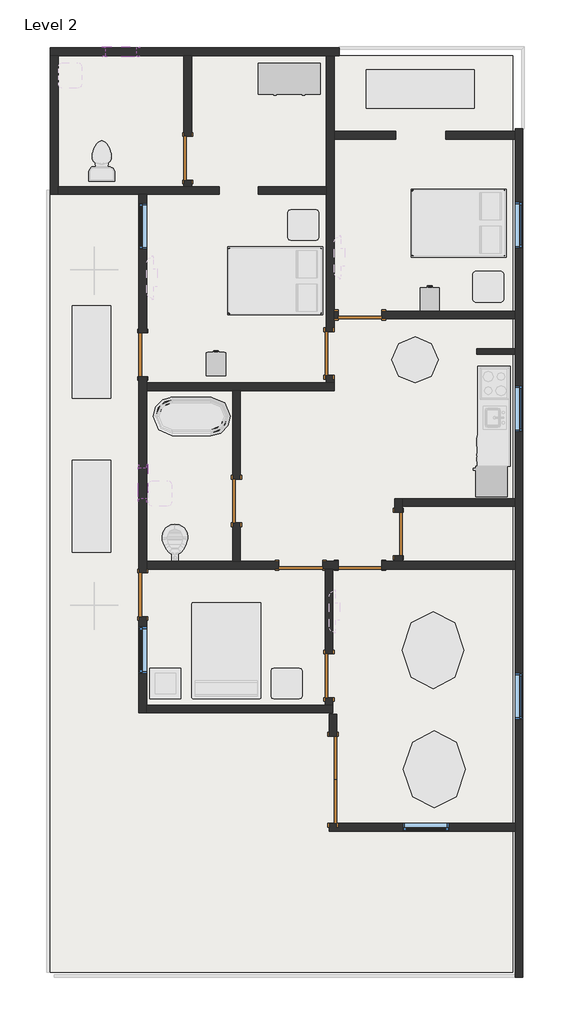
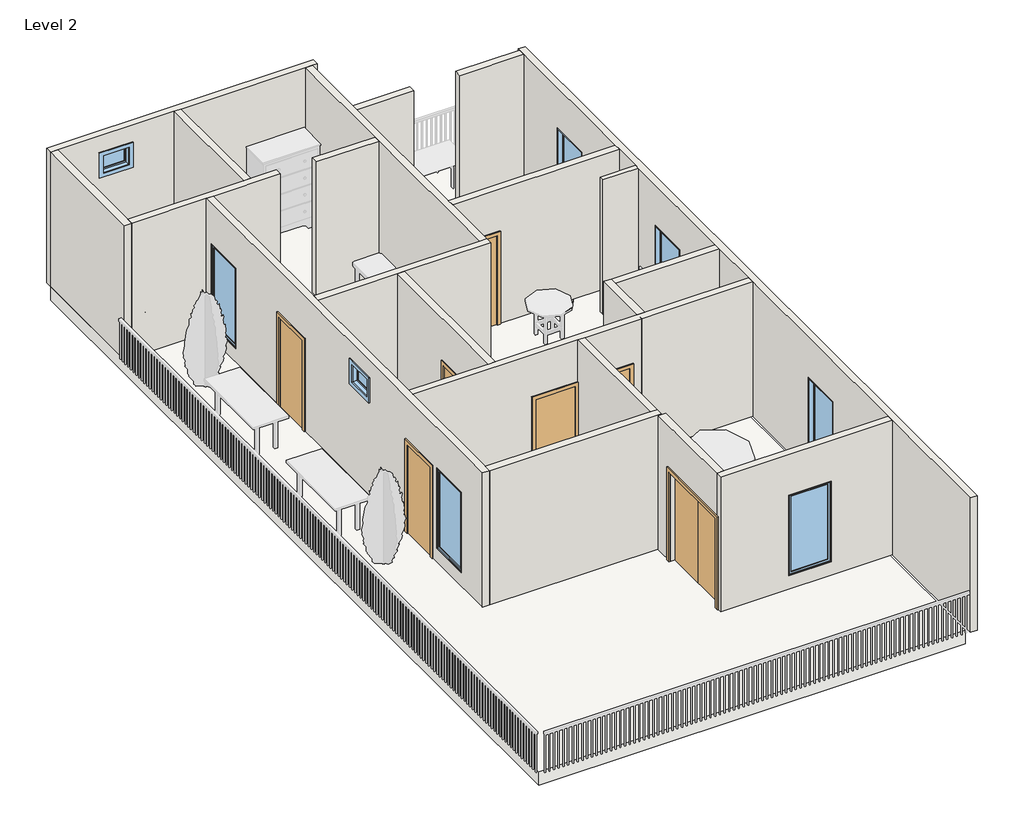
# One storey, part 1 of 4: 22 walls, 11 doors, 8 windows, 1 slab.
"""IFC4 building model written with IfcOpenShell, lengths in millimetres."""

from ifc_helpers import new_model, si_unit, frame, origin, place, context, project, spatial, polyline, outline, extrude, faceted_brep, transform, mapped, element, save
from components import door_74777eb6, door_56e8e0a9, door_706f0888, window_c05a16fb, window_8f6a5eb6

model = new_model("IFC4")

# Units and contexts
model_context = context("Model", 3, world=origin())
ifc_project = project(units=[si_unit("LENGTHUNIT", "METRE", prefix="MILLI")], contexts=[model_context])

# Site, building, storey
site = spatial("IfcSite", under=ifc_project)
building = spatial("IfcBuilding", under=site)
storey = spatial("IfcBuildingStorey", under=building, Name="Level 2", Elevation=3048.0)

# Doors
placement = place(None, origin())
door_shape = door_74777eb6(model_context)
element("IfcDoor", 1, ObjectType="Door-Double-Flush_Panel : 68\" x 80\"", at=placement, inside=storey, context=model_context, shape_type="MappedRepresentation", body=[
    mapped(door_shape, transform((-6447.060887, -797.8089531, 3048.0), x_axis=(0.0, -1.0, 0.0), y_axis=(1.0, 0.0, 0.0), z_axis=(0.0, 0.0, 1.0))),
])
door_2_shape = door_56e8e0a9(model_context)
element("IfcDoor", 2, ObjectType="Single-Flush : 34\" x 80\"", at=placement, inside=storey, context=model_context, shape_type="MappedRepresentation", body=[
    mapped(door_2_shape, transform((-5913.660887, 8396.9910469, 3048.0), x_axis=(-1.0, 0.0, 0.0), y_axis=(0.0, -1.0, 0.0), z_axis=(0.0, 0.0, 1.0))),
])
element("IfcDoor", 3, ObjectType="Single-Flush : 34\" x 80\"", at=placement, inside=storey, context=model_context, shape_type="MappedRepresentation", body=[
    mapped(door_2_shape, transform((-10206.260887, 2859.7910469, 3048.0), x_axis=(0.0, 1.0, 0.0), y_axis=(-1.0, 0.0, 0.0), z_axis=(0.0, 0.0, 1.0))),
])
element("IfcDoor", 4, ObjectType="Single-Flush : 34\" x 80\"", at=placement, inside=storey, context=model_context, shape_type="MappedRepresentation", body=[
    mapped(door_2_shape, transform((-5151.660887, 4066.2910469, 3048.0), x_axis=(0.0, -1.0, 0.0), y_axis=(1.0, 0.0, 0.0), z_axis=(0.0, 0.0, 1.0))),
])
element("IfcDoor", 5, ObjectType="Single-Flush : 34\" x 80\"", at=placement, inside=storey, context=model_context, shape_type="MappedRepresentation", body=[
    mapped(door_2_shape, transform((-5913.660887, 3443.9910469, 3048.0), x_axis=(-1.0, 0.0, 0.0), y_axis=(0.0, -1.0, 0.0), z_axis=(0.0, 0.0, 1.0))),
])
door_3_shape = door_706f0888(model_context)
element("IfcDoor", 6, ObjectType="Single-Flush : 34\" x 80\"", at=placement, inside=storey, context=model_context, shape_type="MappedRepresentation", body=[
    mapped(door_3_shape, transform((-9317.260887, 11495.7910469, 3048.0), x_axis=(0.0, -1.0, 0.0), y_axis=(1.0, 0.0, 0.0), z_axis=(0.0, 0.0, 1.0))),
])
element("IfcDoor", 7, ObjectType="Single-Flush : 34\" x 80\"", at=placement, inside=storey, context=model_context, shape_type="MappedRepresentation", body=[
    mapped(door_3_shape, transform((-6523.260887, 7634.9910469, 3048.0), x_axis=(0.0, -1.0, 0.0), y_axis=(1.0, 0.0, 0.0), z_axis=(0.0, 0.0, 1.0))),
])
element("IfcDoor", 8, ObjectType="Single-Flush : 34\" x 80\"", at=placement, inside=storey, context=model_context, shape_type="MappedRepresentation", body=[
    mapped(door_3_shape, transform((-8352.060887, 4713.9910469, 3048.0), x_axis=(0.0, -1.0, 0.0), y_axis=(1.0, 0.0, 0.0), z_axis=(0.0, 0.0, 1.0))),
])
element("IfcDoor", 9, ObjectType="Single-Flush : 34\" x 80\"", at=placement, inside=storey, context=model_context, shape_type="MappedRepresentation", body=[
    mapped(door_3_shape, transform((-7082.060887, 3443.9910469, 3048.0), x_axis=(1.0, 0.0, 0.0), y_axis=(0.0, 1.0, 0.0), z_axis=(0.0, 0.0, 1.0))),
])
element("IfcDoor", 10, ObjectType="Single-Flush : 34\" x 80\"", at=placement, inside=storey, context=model_context, shape_type="MappedRepresentation", body=[
    mapped(door_3_shape, transform((-10206.260887, 7609.5910469, 3048.0), x_axis=(0.0, -1.0, 0.0), y_axis=(1.0, 0.0, 0.0), z_axis=(0.0, 0.0, 1.0))),
])
element("IfcDoor", 11, ObjectType="Single-Flush : 34\" x 80\"", at=placement, inside=storey, context=model_context, shape_type="MappedRepresentation", body=[
    mapped(door_3_shape, transform((-6523.260887, 1259.5910469, 3048.0), x_axis=(0.0, -1.0, 0.0), y_axis=(1.0, 0.0, 0.0), z_axis=(0.0, 0.0, 1.0))),
])

# Slab
element("IfcSlab", 12, ObjectType="Generic - 12\"", at=placement, inside=storey, context=model_context, shape_type="SweptSolid", body=[
    extrude(outline(polyline([(-2891.060887, 13527.7910469), (-2891.060887, -4607.8089531), (-12035.060887, -4607.8089531), (-12035.060887, 13527.7910469), (-2891.060887, 13527.7910469)])), frame((0.0, 0.0, 2743.2), z_axis=(0.0, 0.0, 1.0), x_axis=(1.0, 0.0, 0.0)), (0.0, 0.0, 1.0), 304.8),
])

# Walls
element("IfcWall", 13, ObjectType="Generic - 8\"", at=placement, inside=storey, context=model_context, shape_type="Brep", body=[
    faceted_brep([(-12035.060887, 13527.7910469, 3048.0), (-11882.660887, 13527.7910469, 3048.0), (-9393.460887, 13527.7910469, 3048.0), (-9241.060887, 13527.7910469, 3048.0), (-6574.060887, 13527.7910469, 3048.0), (-6421.660887, 13527.7910469, 3048.0), (-6320.060887, 13527.7910469, 3048.0), (-6320.060887, 13527.7910469, 6096.0), (-6421.660887, 13527.7910469, 6096.0), (-6574.060887, 13527.7910469, 6096.0), (-9241.060887, 13527.7910469, 6096.0), (-9393.460887, 13527.7910469, 6096.0), (-11882.660887, 13527.7910469, 6096.0), (-12035.060887, 13527.7910469, 6096.0), (-10333.260887, 13527.7910469, 5664.2), (-10333.260887, 13527.7910469, 5207.0), (-10942.860887, 13527.7910469, 5207.0), (-10942.860887, 13527.7910469, 5664.2), (-12035.060887, 13680.1910469, 3048.0), (-12035.060887, 13680.1910469, 6096.0), (-6320.060887, 13680.1910469, 6096.0), (-6320.060887, 13680.1910469, 3048.0), (-10333.260887, 13680.1910469, 5664.2), (-10942.860887, 13680.1910469, 5664.2), (-10942.860887, 13680.1910469, 5207.0), (-10333.260887, 13680.1910469, 5207.0)], [[[0, 1, 2, 3, 4, 5, 6, 7, 8, 9, 10, 11, 12, 13], [14, 15, 16, 17]], [[18, 19, 20, 21], [22, 23, 24, 25]], [[6, 5, 4, 3, 2, 1, 0, 18, 21]], [[7, 6, 21, 20]], [[13, 12, 11, 10, 9, 8, 7, 20, 19]], [[0, 13, 19, 18]], [[15, 14, 22, 25]], [[16, 15, 25, 24]], [[17, 16, 24, 23]], [[14, 17, 23, 22]]]),
])
element("IfcWall", 14, ObjectType="Generic - 8\"", at=placement, inside=storey, context=model_context, shape_type="Brep", body=[
    faceted_brep([(-12035.060887, 13527.7910469, 3048.0), (-12035.060887, 10784.5910469, 3048.0), (-12035.060887, 10784.5910469, 6096.0), (-12035.060887, 13527.7910469, 6096.0), (-11882.660887, 13527.7910469, 3048.0), (-11882.660887, 13527.7910469, 6096.0), (-11882.660887, 10936.9910469, 6096.0), (-11882.660887, 10784.5910469, 6096.0), (-11882.660887, 10784.5910469, 3048.0), (-11882.660887, 10936.9910469, 3048.0)], [[[0, 1, 2, 3]], [[4, 5, 6, 7, 8, 9]], [[1, 0, 4, 9, 8]], [[3, 2, 7, 6, 5]], [[0, 3, 5, 4]], [[2, 1, 8, 7]]]),
])
element("IfcWall", 15, ObjectType="Generic - 8\"", at=placement, inside=storey, context=model_context, shape_type="Brep", body=[
    faceted_brep([(-11882.660887, 10784.5910469, 3048.0), (-10282.460887, 10784.5910469, 3048.0), (-10130.060887, 10784.5910469, 3048.0), (-8694.960887, 10784.5910469, 3048.0), (-8694.960887, 10784.5910469, 6096.0), (-10130.060887, 10784.5910469, 6096.0), (-10282.460887, 10784.5910469, 6096.0), (-11882.660887, 10784.5910469, 6096.0), (-11882.660887, 10936.9910469, 3048.0), (-11882.660887, 10936.9910469, 6096.0), (-9393.460887, 10936.9910469, 6096.0), (-9241.060887, 10936.9910469, 6096.0), (-8694.960887, 10936.9910469, 6096.0), (-8694.960887, 10936.9910469, 3048.0), (-9241.060887, 10936.9910469, 3048.0), (-9393.460887, 10936.9910469, 3048.0)], [[[0, 1, 2, 3, 4, 5, 6, 7]], [[8, 9, 10, 11, 12, 13, 14, 15]], [[3, 2, 1, 0, 8, 15, 14, 13]], [[4, 3, 13, 12]], [[7, 6, 5, 4, 12, 11, 10, 9]], [[0, 7, 9, 8]]]),
])
element("IfcWall", 16, ObjectType="Generic - 8\"", at=placement, inside=storey, context=model_context, shape_type="Brep", body=[
    faceted_brep([(-10282.460887, 522.9910469, 6096.0), (-10282.460887, 10784.5910469, 6096.0), (-10282.460887, 10784.5910469, 3048.0), (-10282.460887, 8041.3910469, 3048.0), (-10282.460887, 8041.3910469, 5080.0), (-10282.460887, 7177.7910469, 5080.0), (-10282.460887, 7177.7910469, 3048.0), (-10282.460887, 3291.5910469, 3048.0), (-10282.460887, 3291.5910469, 5080.0), (-10282.460887, 2427.9910469, 5080.0), (-10282.460887, 2427.9910469, 3048.0), (-10282.460887, 522.9910469, 3048.0), (-10282.460887, 10606.7910469, 3352.8), (-10282.460887, 10606.7910469, 5181.6), (-10282.460887, 9692.3910469, 5181.6), (-10282.460887, 9692.3910469, 3352.8), (-10282.460887, 2224.7910469, 3352.8), (-10282.460887, 2224.7910469, 5181.6), (-10282.460887, 1310.3910469, 5181.6), (-10282.460887, 1310.3910469, 3352.8), (-10282.460887, 4764.7910469, 5664.2), (-10282.460887, 4764.7910469, 5207.0), (-10282.460887, 5374.3910469, 5207.0), (-10282.460887, 5374.3910469, 5664.2), (-10130.060887, 10784.5910469, 6096.0), (-10130.060887, 7050.7910469, 6096.0), (-10130.060887, 6898.3910469, 6096.0), (-10130.060887, 3520.1910469, 6096.0), (-10130.060887, 3367.7910469, 6096.0), (-10130.060887, 675.3910469, 6096.0), (-10130.060887, 522.9910469, 6096.0), (-10130.060887, 522.9910469, 3048.0), (-10130.060887, 675.3910469, 3048.0), (-10130.060887, 2427.9910469, 3048.0), (-10130.060887, 2427.9910469, 5080.0), (-10130.060887, 3291.5910469, 5080.0), (-10130.060887, 3291.5910469, 3048.0), (-10130.060887, 3367.7910469, 3048.0), (-10130.060887, 3520.1910469, 3048.0), (-10130.060887, 6898.3910469, 3048.0), (-10130.060887, 7050.7910469, 3048.0), (-10130.060887, 7177.7910469, 3048.0), (-10130.060887, 7177.7910469, 5080.0), (-10130.060887, 8041.3910469, 5080.0), (-10130.060887, 8041.3910469, 3048.0), (-10130.060887, 10784.5910469, 3048.0), (-10130.060887, 10606.7910469, 5181.6), (-10130.060887, 10606.7910469, 3352.8), (-10130.060887, 9692.3910469, 3352.8), (-10130.060887, 9692.3910469, 5181.6), (-10130.060887, 2224.7910469, 5181.6), (-10130.060887, 2224.7910469, 3352.8), (-10130.060887, 1310.3910469, 3352.8), (-10130.060887, 1310.3910469, 5181.6), (-10130.060887, 4764.7910469, 5207.0), (-10130.060887, 4764.7910469, 5664.2), (-10130.060887, 5374.3910469, 5664.2), (-10130.060887, 5374.3910469, 5207.0)], [[[0, 1, 2, 3, 4, 5, 6, 7, 8, 9, 10, 11], [12, 13, 14, 15], [16, 17, 18, 19], [20, 21, 22, 23]], [[24, 25, 26, 27, 28, 29, 30, 31, 32, 33, 34, 35, 36, 37, 38, 39, 40, 41, 42, 43, 44, 45], [46, 47, 48, 49], [50, 51, 52, 53], [54, 55, 56, 57]], [[2, 45, 44, 3]], [[31, 11, 10, 33, 32]], [[6, 41, 40, 39, 38, 37, 36, 7]], [[1, 0, 30, 29, 28, 27, 26, 25, 24]], [[2, 1, 24, 45]], [[0, 11, 31, 30]], [[12, 47, 46, 13]], [[47, 12, 15, 48]], [[48, 15, 14, 49]], [[50, 17, 16, 51]], [[51, 16, 19, 52]], [[52, 19, 18, 53]], [[13, 46, 49, 14]], [[17, 50, 53, 18]], [[21, 20, 55, 54]], [[22, 21, 54, 57]], [[23, 22, 57, 56]], [[20, 23, 56, 55]], [[42, 41, 6, 5]], [[43, 42, 5, 4]], [[44, 43, 4, 3]], [[35, 8, 7, 36]], [[8, 35, 34, 9]], [[10, 9, 34, 33]]]),
])
element("IfcWall", 17, ObjectType="Generic - 8\"", at=placement, inside=storey, context=model_context, shape_type="Brep", body=[
    faceted_brep([(-10130.060887, 6898.3910469, 3048.0), (-8428.260887, 6898.3910469, 3048.0), (-8275.860887, 6898.3910469, 3048.0), (-6421.660887, 6898.3910469, 3048.0), (-6421.660887, 6898.3910469, 6096.0), (-8275.860887, 6898.3910469, 6096.0), (-8428.260887, 6898.3910469, 6096.0), (-10130.060887, 6898.3910469, 6096.0), (-10130.060887, 7050.7910469, 3048.0), (-10130.060887, 7050.7910469, 6096.0), (-6574.060887, 7050.7910469, 6096.0), (-6421.660887, 7050.7910469, 6096.0), (-6421.660887, 7050.7910469, 3048.0), (-6574.060887, 7050.7910469, 3048.0)], [[[0, 1, 2, 3, 4, 5, 6, 7]], [[8, 9, 10, 11, 12, 13]], [[3, 2, 1, 0, 8, 13, 12]], [[7, 6, 5, 4, 11, 10, 9]], [[0, 7, 9, 8]], [[4, 3, 12, 11]]]),
])
element("IfcWall", 18, ObjectType="Generic - 8\"", at=placement, inside=storey, context=model_context, shape_type="Brep", body=[
    faceted_brep([(-6421.660887, 13527.7910469, 6096.0), (-6421.660887, 12029.1910469, 6096.0), (-6421.660887, 11876.7910469, 6096.0), (-6421.660887, 8473.1910469, 6096.0), (-6421.660887, 8320.7910469, 6096.0), (-6421.660887, 7050.7910469, 6096.0), (-6421.660887, 7050.7910469, 3048.0), (-6421.660887, 7203.1910469, 3048.0), (-6421.660887, 7203.1910469, 5080.0), (-6421.660887, 8066.7910469, 5080.0), (-6421.660887, 8066.7910469, 3048.0), (-6421.660887, 8320.7910469, 3048.0), (-6421.660887, 8473.1910469, 3048.0), (-6421.660887, 11876.7910469, 3048.0), (-6421.660887, 12029.1910469, 3048.0), (-6421.660887, 13527.7910469, 3048.0), (-6574.060887, 7050.7910469, 6096.0), (-6574.060887, 10784.5910469, 6096.0), (-6574.060887, 10936.9910469, 6096.0), (-6574.060887, 13527.7910469, 6096.0), (-6574.060887, 13527.7910469, 3048.0), (-6574.060887, 10936.9910469, 3048.0), (-6574.060887, 10784.5910469, 3048.0), (-6574.060887, 8066.7910469, 3048.0), (-6574.060887, 8066.7910469, 5080.0), (-6574.060887, 7203.1910469, 5080.0), (-6574.060887, 7203.1910469, 3048.0), (-6574.060887, 7050.7910469, 3048.0)], [[[0, 1, 2, 3, 4, 5, 6, 7, 8, 9, 10, 11, 12, 13, 14, 15]], [[16, 17, 18, 19, 20, 21, 22, 23, 24, 25, 26, 27]], [[6, 27, 26, 7]], [[20, 15, 14, 13, 12, 11, 10, 23, 22, 21]], [[5, 4, 3, 2, 1, 0, 19, 18, 17, 16]], [[6, 5, 16, 27]], [[0, 15, 20, 19]], [[25, 8, 7, 26]], [[8, 25, 24, 9]], [[9, 24, 23, 10]]]),
])
element("IfcWall", 19, ObjectType="Generic - 8\"", at=placement, inside=storey, context=model_context, shape_type="SweptSolid", body=[
    extrude(outline(polyline([(-5202.460887, 11876.7910469), (-6421.660887, 11876.7910469), (-6421.660887, 12029.1910469), (-5202.460887, 12029.1910469), (-5202.460887, 11876.7910469)])), frame((0.0, 0.0, 3048.0), z_axis=(0.0, 0.0, 1.0), x_axis=(1.0, 0.0, 0.0)), (0.0, 0.0, 1.0), 3048.0),
])
element("IfcWall", 20, ObjectType="Generic - 8\"", at=placement, inside=storey, context=model_context, shape_type="SweptSolid", body=[
    extrude(outline(polyline([(3048.0, -6421.660887), (3048.0, -6345.460887), (5080.0, -6345.460887), (5080.0, -5481.860887), (3048.0, -5481.860887), (3048.0, -2840.260887), (6096.0, -2840.260887), (6096.0, -6421.660887), (3048.0, -6421.660887)])), frame((0.0, 8320.7910469, 0.0), z_axis=(0.0, 1.0, 0.0), x_axis=(0.0, 0.0, 1.0)), (0.0, 0.0, 1.0), 152.4),
])
element("IfcWall", 21, ObjectType="Generic - 8\"", at=placement, inside=storey, context=model_context, shape_type="Brep", body=[
    faceted_brep([(-10130.060887, 522.9910469, 3048.0), (-6447.060887, 522.9910469, 3048.0), (-6447.060887, 522.9910469, 6096.0), (-10130.060887, 522.9910469, 6096.0), (-10130.060887, 675.3910469, 3048.0), (-10130.060887, 675.3910469, 6096.0), (-6599.460887, 675.3910469, 6096.0), (-6447.060887, 675.3910469, 6096.0), (-6447.060887, 675.3910469, 3048.0), (-6599.460887, 675.3910469, 3048.0)], [[[0, 1, 2, 3]], [[4, 5, 6, 7, 8, 9]], [[1, 0, 4, 9, 8]], [[3, 2, 7, 6, 5]], [[0, 3, 5, 4]], [[2, 1, 8, 7]]]),
])
element("IfcWall", 22, ObjectType="Generic - 8\"", at=placement, inside=storey, context=model_context, shape_type="SweptSolid", body=[
    extrude(outline(polyline([(827.7910469, 5080.0), (827.7910469, 3048.0), (675.3910469, 3048.0), (675.3910469, 6096.0), (3367.7910469, 6096.0), (3367.7910469, 3048.0), (1691.3910469, 3048.0), (1691.3910469, 5080.0), (827.7910469, 5080.0)])), frame((-6599.460887, 0.0, 0.0), z_axis=(1.0, 0.0, 0.0), x_axis=(0.0, 1.0, 0.0)), (0.0, 0.0, 1.0), 152.4),
])
element("IfcWall", 23, ObjectType="Generic - 8\"", at=placement, inside=storey, context=model_context, shape_type="Brep", body=[
    faceted_brep([(-6345.460887, 3520.1910469, 5080.0), (-6345.460887, 3520.1910469, 3048.0), (-6650.260887, 3520.1910469, 3048.0), (-6650.260887, 3520.1910469, 5080.0), (-7513.860887, 3520.1910469, 5080.0), (-7513.860887, 3520.1910469, 3048.0), (-8275.860887, 3520.1910469, 3048.0), (-8428.260887, 3520.1910469, 3048.0), (-10130.060887, 3520.1910469, 3048.0), (-10130.060887, 3520.1910469, 6096.0), (-8428.260887, 3520.1910469, 6096.0), (-8275.860887, 3520.1910469, 6096.0), (-2840.260887, 3520.1910469, 6096.0), (-2840.260887, 3520.1910469, 3048.0), (-5481.860887, 3520.1910469, 3048.0), (-5481.860887, 3520.1910469, 5080.0), (-6650.260887, 3367.7910469, 3048.0), (-6599.460887, 3367.7910469, 3048.0), (-6447.060887, 3367.7910469, 3048.0), (-6345.460887, 3367.7910469, 3048.0), (-6345.460887, 3367.7910469, 5080.0), (-5481.860887, 3367.7910469, 5080.0), (-5481.860887, 3367.7910469, 3048.0), (-2840.260887, 3367.7910469, 3048.0), (-2840.260887, 3367.7910469, 6096.0), (-6447.060887, 3367.7910469, 6096.0), (-6599.460887, 3367.7910469, 6096.0), (-10130.060887, 3367.7910469, 6096.0), (-10130.060887, 3367.7910469, 3048.0), (-7513.860887, 3367.7910469, 3048.0), (-7513.860887, 3367.7910469, 5080.0), (-6650.260887, 3367.7910469, 5080.0)], [[[0, 1, 2, 3, 4, 5, 6, 7, 8, 9, 10, 11, 12, 13, 14, 15]], [[16, 17, 18, 19, 20, 21, 22, 23, 24, 25, 26, 27, 28, 29, 30, 31]], [[29, 28, 8, 7, 6, 5]], [[14, 13, 23, 22]], [[2, 1, 19, 18, 17, 16]], [[12, 11, 10, 9, 27, 26, 25, 24]], [[9, 8, 28, 27]], [[13, 12, 24, 23]], [[3, 2, 16, 31]], [[4, 3, 31, 30]], [[5, 4, 30, 29]], [[20, 19, 1, 0]], [[21, 20, 0, 15]], [[22, 21, 15, 14]]]),
])
element("IfcWall", 24, ObjectType="Generic - 8\"", at=placement, inside=storey, context=model_context, shape_type="SweptSolid", body=[
    extrude(outline(polyline([(4282.1910469, 5080.0), (4282.1910469, 3048.0), (3520.1910469, 3048.0), (3520.1910469, 6096.0), (6898.3910469, 6096.0), (6898.3910469, 3048.0), (5145.7910469, 3048.0), (5145.7910469, 5080.0), (4282.1910469, 5080.0)])), frame((-8428.260887, 0.0, 0.0), z_axis=(1.0, 0.0, 0.0), x_axis=(0.0, 1.0, 0.0)), (0.0, 0.0, 1.0), 152.4),
])
element("IfcWall", 25, ObjectType="Generic - 8\"", at=placement, inside=storey, context=model_context, shape_type="Brep", body=[
    faceted_brep([(-6523.260887, -1813.8089531, 3048.0), (-2840.260887, -1813.8089531, 3048.0), (-2840.260887, -1813.8089531, 6096.0), (-6523.260887, -1813.8089531, 6096.0), (-5062.760887, -1813.8089531, 3352.8), (-5062.760887, -1813.8089531, 5181.6), (-4148.360887, -1813.8089531, 5181.6), (-4148.360887, -1813.8089531, 3352.8), (-2840.260887, -1661.4089531, 3048.0), (-6523.260887, -1661.4089531, 3048.0), (-6523.260887, -1661.4089531, 5080.0), (-6523.260887, -1661.4089531, 6096.0), (-6370.860887, -1661.4089531, 6096.0), (-2840.260887, -1661.4089531, 6096.0), (-5062.760887, -1661.4089531, 5181.6), (-5062.760887, -1661.4089531, 3352.8), (-4148.360887, -1661.4089531, 3352.8), (-4148.360887, -1661.4089531, 5181.6)], [[[0, 1, 2, 3], [4, 5, 6, 7]], [[8, 9, 10, 11, 12, 13], [14, 15, 16, 17]], [[1, 0, 9, 8]], [[3, 2, 13, 12, 11]], [[2, 1, 8, 13]], [[0, 3, 11, 10, 9]], [[14, 5, 4, 15]], [[15, 4, 7, 16]], [[16, 7, 6, 17]], [[5, 14, 17, 6]]]),
])
element("IfcWall", 26, ObjectType="Generic - 8\"", at=placement, inside=storey, context=model_context, shape_type="SweptSolid", body=[
    extrude(outline(polyline([(497.5910469, 6096.0), (497.5910469, 3048.0), (65.7910469, 3048.0), (65.7910469, 5080.0), (-1661.4089531, 5080.0), (-1661.4089531, 6096.0), (497.5910469, 6096.0)])), frame((-6523.260887, 0.0, 0.0), z_axis=(1.0, 0.0, 0.0), x_axis=(0.0, 1.0, 0.0)), (0.0, 0.0, 1.0), 152.4),
])
element("IfcWall", 27, ObjectType="Generic - 8\"", at=placement, inside=storey, context=model_context, shape_type="Brep", body=[
    faceted_brep([(-2840.260887, 3520.1910469, 3048.0), (-5075.460887, 3520.1910469, 3048.0), (-5227.860887, 3520.1910469, 3048.0), (-5227.860887, 3520.1910469, 6096.0), (-5075.460887, 3520.1910469, 6096.0), (-2840.260887, 3520.1910469, 6096.0), (-2840.260887, 3367.7910469, 3048.0), (-2840.260887, 3367.7910469, 6096.0), (-5227.860887, 3367.7910469, 6096.0), (-5227.860887, 3367.7910469, 3048.0)], [[[0, 1, 2, 3, 4, 5]], [[6, 7, 8, 9]], [[2, 1, 0, 6, 9]], [[5, 4, 3, 8, 7]], [[0, 5, 7, 6]], [[3, 2, 9, 8]]]),
])
element("IfcWall", 28, ObjectType="Generic - 8\"", at=placement, inside=storey, context=model_context, shape_type="Brep", body=[
    faceted_brep([(-5075.460887, 3520.1910469, 3048.0), (-5075.460887, 3634.4910469, 3048.0), (-5075.460887, 3634.4910469, 5080.0), (-5075.460887, 4498.0910469, 5080.0), (-5075.460887, 4498.0910469, 3048.0), (-5075.460887, 4612.3910469, 3048.0), (-5075.460887, 4764.7910469, 3048.0), (-5075.460887, 4764.7910469, 6096.0), (-5075.460887, 4612.3910469, 6096.0), (-5075.460887, 3520.1910469, 6096.0), (-5227.860887, 3634.4910469, 5080.0), (-5227.860887, 3634.4910469, 3048.0), (-5227.860887, 3520.1910469, 3048.0), (-5227.860887, 3520.1910469, 6096.0), (-5227.860887, 4764.7910469, 6096.0), (-5227.860887, 4764.7910469, 3048.0), (-5227.860887, 4498.0910469, 3048.0), (-5227.860887, 4498.0910469, 5080.0)], [[[0, 1, 2, 3, 4, 5, 6, 7, 8, 9]], [[10, 11, 12, 13, 14, 15, 16, 17]], [[16, 15, 6, 5, 4]], [[12, 11, 1, 0]], [[9, 8, 7, 14, 13]], [[0, 9, 13, 12]], [[7, 6, 15, 14]], [[2, 1, 11, 10]], [[3, 2, 10, 17]], [[4, 3, 17, 16]]]),
])
element("IfcWall", 29, ObjectType="Generic - 8\"", at=placement, inside=storey, context=model_context, shape_type="SweptSolid", body=[
    extrude(outline(polyline([(-2840.260887, 4612.3910469), (-5075.460887, 4612.3910469), (-5075.460887, 4764.7910469), (-2840.260887, 4764.7910469), (-2840.260887, 4612.3910469)])), frame((0.0, 0.0, 3048.0), z_axis=(0.0, 0.0, 1.0), x_axis=(1.0, 0.0, 0.0)), (0.0, 0.0, 1.0), 3048.0),
])
element("IfcWall", 30, ObjectType="Generic - 8\"", at=placement, inside=storey, context=model_context, shape_type="SweptSolid", body=[
    extrude(outline(polyline([(10936.9910469, 6096.0), (13527.7910469, 6096.0), (13527.7910469, 3048.0), (11927.5910469, 3048.0), (11927.5910469, 5080.0), (11063.9910469, 5080.0), (11063.9910469, 3048.0), (10936.9910469, 3048.0), (10936.9910469, 6096.0)])), frame((-9393.460887, 0.0, 0.0), z_axis=(1.0, 0.0, 0.0), x_axis=(0.0, 1.0, 0.0)), (0.0, 0.0, 1.0), 152.4),
])
element("IfcWall", 31, ObjectType="Generic - 8\"", at=placement, inside=storey, context=model_context, shape_type="SweptSolid", body=[
    extrude(outline(polyline([(-6574.060887, 10784.5910469), (-7920.260887, 10784.5910469), (-7920.260887, 10936.9910469), (-6574.060887, 10936.9910469), (-6574.060887, 10784.5910469)])), frame((0.0, 0.0, 3048.0), z_axis=(0.0, 0.0, 1.0), x_axis=(1.0, 0.0, 0.0)), (0.0, 0.0, 1.0), 3048.0),
])
element("IfcWall", 32, ObjectType="Generic - 8\"", at=placement, inside=storey, context=model_context, shape_type="SweptSolid", body=[
    extrude(outline(polyline([(-2840.260887, 11876.7910469), (-4211.860887, 11876.7910469), (-4211.860887, 12029.1910469), (-2840.260887, 12029.1910469), (-2840.260887, 11876.7910469)])), frame((0.0, 0.0, 3048.0), z_axis=(0.0, 0.0, 1.0), x_axis=(1.0, 0.0, 0.0)), (0.0, 0.0, 1.0), 3048.0),
])
element("IfcWall", 33, ObjectType="Generic - 8\"", at=placement, inside=storey, context=model_context, shape_type="Brep", body=[
    faceted_brep([(-2840.260887, 12079.9910469, 3048.0), (-2840.260887, 12029.1910469, 3048.0), (-2840.260887, 11876.7910469, 3048.0), (-2840.260887, 8473.1910469, 3048.0), (-2840.260887, 8320.7910469, 3048.0), (-2840.260887, 7723.8910469, 3048.0), (-2840.260887, 7622.2910469, 3048.0), (-2840.260887, 4764.7910469, 3048.0), (-2840.260887, 4612.3910469, 3048.0), (-2840.260887, 3520.1910469, 3048.0), (-2840.260887, 3367.7910469, 3048.0), (-2840.260887, -1661.4089531, 3048.0), (-2840.260887, -1813.8089531, 3048.0), (-2840.260887, -4709.4089531, 3048.0), (-2840.260887, -4709.4089531, 6096.0), (-2840.260887, -1813.8089531, 6096.0), (-2840.260887, -1661.4089531, 6096.0), (-2840.260887, 3367.7910469, 6096.0), (-2840.260887, 3520.1910469, 6096.0), (-2840.260887, 4612.3910469, 6096.0), (-2840.260887, 4764.7910469, 6096.0), (-2840.260887, 7622.2910469, 6096.0), (-2840.260887, 7723.8910469, 6096.0), (-2840.260887, 8320.7910469, 6096.0), (-2840.260887, 8473.1910469, 6096.0), (-2840.260887, 11876.7910469, 6096.0), (-2840.260887, 12029.1910469, 6096.0), (-2840.260887, 12079.9910469, 6096.0), (-2840.260887, 9717.7910469, 5181.6), (-2840.260887, 9717.7910469, 3352.8), (-2840.260887, 10632.1910469, 3352.8), (-2840.260887, 10632.1910469, 5181.6), (-2840.260887, 6085.5910469, 5181.6), (-2840.260887, 6085.5910469, 3352.8), (-2840.260887, 6999.9910469, 3352.8), (-2840.260887, 6999.9910469, 5181.6), (-2840.260887, 395.9910469, 5181.6), (-2840.260887, 395.9910469, 3352.8), (-2840.260887, 1310.3910469, 3352.8), (-2840.260887, 1310.3910469, 5181.6), (-2687.860887, -4709.4089531, 3048.0), (-2687.860887, 12079.9910469, 3048.0), (-2687.860887, 12079.9910469, 6096.0), (-2687.860887, -4709.4089531, 6096.0), (-2687.860887, 9717.7910469, 3352.8), (-2687.860887, 9717.7910469, 5181.6), (-2687.860887, 10632.1910469, 5181.6), (-2687.860887, 10632.1910469, 3352.8), (-2687.860887, 6085.5910469, 3352.8), (-2687.860887, 6085.5910469, 5181.6), (-2687.860887, 6999.9910469, 5181.6), (-2687.860887, 6999.9910469, 3352.8), (-2687.860887, 395.9910469, 3352.8), (-2687.860887, 395.9910469, 5181.6), (-2687.860887, 1310.3910469, 5181.6), (-2687.860887, 1310.3910469, 3352.8)], [[[0, 1, 2, 3, 4, 5, 6, 7, 8, 9, 10, 11, 12, 13, 14, 15, 16, 17, 18, 19, 20, 21, 22, 23, 24, 25, 26, 27], [28, 29, 30, 31], [32, 33, 34, 35], [36, 37, 38, 39]], [[40, 41, 42, 43], [44, 45, 46, 47], [48, 49, 50, 51], [52, 53, 54, 55]], [[13, 12, 11, 10, 9, 8, 7, 6, 5, 4, 3, 2, 1, 0, 41, 40]], [[14, 13, 40, 43]], [[27, 26, 25, 24, 23, 22, 21, 20, 19, 18, 17, 16, 15, 14, 43, 42]], [[0, 27, 42, 41]], [[44, 29, 28, 45]], [[29, 44, 47, 30]], [[30, 47, 46, 31]], [[48, 33, 32, 49]], [[33, 48, 51, 34]], [[34, 51, 50, 35]], [[36, 53, 52, 37]], [[37, 52, 55, 38]], [[38, 55, 54, 39]], [[45, 28, 31, 46]], [[49, 32, 35, 50]], [[53, 36, 39, 54]]]),
])
element("IfcWall", 34, ObjectType="WALL 4\"", at=placement, inside=storey, context=model_context, shape_type="SweptSolid", body=[
    extrude(outline(polyline([(-3602.260887, 7723.8910469), (-2840.260887, 7723.8910469), (-2840.260887, 7622.2910469), (-3602.260887, 7622.2910469), (-3602.260887, 7723.8910469)])), frame((0.0, 0.0, 3048.0), z_axis=(0.0, 0.0, 1.0), x_axis=(1.0, 0.0, 0.0)), (0.0, 0.0, 1.0), 3048.0),
])

# Windows
window_shape = window_c05a16fb(model_context)
element("IfcWindow", 35, ObjectType="Fixed : 36\" x 72\"", at=placement, inside=storey, context=model_context, shape_type="MappedRepresentation", body=[
    mapped(window_shape, transform((-2764.060887, 10136.8910469, 3048.0), x_axis=(0.0, -1.0, 0.0), y_axis=(1.0, 0.0, 0.0), z_axis=(0.0, 0.0, 1.0))),
])
element("IfcWindow", 36, ObjectType="Fixed : 36\" x 72\"", at=placement, inside=storey, context=model_context, shape_type="MappedRepresentation", body=[
    mapped(window_shape, transform((-2764.060887, 6504.6910469, 3048.0), x_axis=(0.0, -1.0, 0.0), y_axis=(1.0, 0.0, 0.0), z_axis=(0.0, 0.0, 1.0))),
])
element("IfcWindow", 37, ObjectType="Fixed : 36\" x 72\"", at=placement, inside=storey, context=model_context, shape_type="MappedRepresentation", body=[
    mapped(window_shape, transform((-2764.060887, 815.0910469, 3048.0), x_axis=(0.0, -1.0, 0.0), y_axis=(1.0, 0.0, 0.0), z_axis=(0.0, 0.0, 1.0))),
])
element("IfcWindow", 38, ObjectType="Fixed : 36\" x 72\"", at=placement, inside=storey, context=model_context, shape_type="MappedRepresentation", body=[
    mapped(window_shape, transform((-4643.660887, -1737.6089531, 3048.0), x_axis=(-1.0, 0.0, 0.0), y_axis=(0.0, -1.0, 0.0), z_axis=(0.0, 0.0, 1.0))),
])
element("IfcWindow", 39, ObjectType="Fixed : 36\" x 72\"", at=placement, inside=storey, context=model_context, shape_type="MappedRepresentation", body=[
    mapped(window_shape, transform((-10206.260887, 1805.6910469, 3048.0), x_axis=(0.0, 1.0, 0.0), y_axis=(-1.0, 0.0, 0.0), z_axis=(0.0, 0.0, 1.0))),
])
element("IfcWindow", 40, ObjectType="Fixed : 36\" x 72\"", at=placement, inside=storey, context=model_context, shape_type="MappedRepresentation", body=[
    mapped(window_shape, transform((-10206.260887, 10187.6910469, 3048.0), x_axis=(0.0, 1.0, 0.0), y_axis=(-1.0, 0.0, 0.0), z_axis=(0.0, 0.0, 1.0))),
])
window_2_shape = window_8f6a5eb6(model_context)
element("IfcWindow", 41, ObjectType="Transom with Trim : 24\" x 18\"", at=placement, inside=storey, context=model_context, shape_type="MappedRepresentation", body=[
    mapped(window_2_shape, transform((-10206.260887, 5031.4910469, 3048.0), x_axis=(0.0, -1.0, 0.0), y_axis=(1.0, 0.0, 0.0), z_axis=(0.0, 0.0, 1.0))),
])
element("IfcWindow", 42, ObjectType="Transom with Trim : 24\" x 18\"", at=placement, inside=storey, context=model_context, shape_type="MappedRepresentation", body=[
    mapped(window_2_shape, transform((-10599.960887, 13603.9910469, 3048.0), x_axis=(1.0, 0.0, 0.0), y_axis=(0.0, 1.0, 0.0), z_axis=(0.0, 0.0, 1.0))),
])

save(model, "model.ifc")

# Revit data of these elements
# Type "Door-Double-Flush_Panel : 68\" x 80\""
#   Type Mark = "8"
#   Construction Type Id = "DOOR"
#   Assembly Code = "C1020"
#   Analytic Construction = "Wooden"
#   Thickness = 0' - 2"
#   Thermal Resistance (R) = 2.5876 (h·ft²·°F)/BTU
#   Swing Angle [instance default] = 90.00°
#   Panel Width = 2' - 10"
#   Heat Transfer Coefficient (U) = 0.3865 BTU/(h·ft²·°F)
#   Height = 6' - 8"
#   Trim Projection Ext = 0' - 1"
#   Trim Projection Int = 0' - 1"
#   Trim Width = 0' - 3"
#   Width = 5' - 8"
#   Define Thermal Properties by = 1
#   Panel Material = Wood - Birch - Solid Stained Light Low Gloss
#   Trim Material = Paint - Sienna
#   Visual Light Transmittance = 0
#   Solar Heat Gain Coefficient = 0
#   Function = (empty or 0)
#   Wall Closure = (empty or 0)
# Type "Single-Flush : 34\" x 80\""
#   Type Mark = "7"
#   Construction Type Id = "MDOOR"
#   Assembly Code = "C1020"
#   Analytic Construction = "Metal"
#   Thickness = 0' - 2"
#   Heat Transfer Coefficient (U) = 0.651978 BTU/(h·ft²·°F)
#   Height = 6' - 8"
#   Trim Projection Ext = 0' - 1"
#   Trim Projection Int = 0' - 1"
#   Trim Width = 0' - 3"
#   Width = 2' - 10"
#   Define Thermal Properties by = 1
#   Door Material = Door - Panel
#   Frame Material = Door - Frame
#   Visual Light Transmittance = 0
#   Solar Heat Gain Coefficient = 0
#   Function = (empty or 0)
#   Wall Closure = (empty or 0)
# Type "Generic - 12\""
#   Assembly Code = "B1010"
#   Function = 0
#   Layers, outside or top first: 1' - 0" no material (function 1)
# Type "Generic - 8\""
#   Assembly Code = "B2010"
#   Layers, outside or top first: 0' - 6" "Brick, Common" (function 1)
# Type "WALL 4\""
#   Assembly Code = "B2010"
#   Layers, outside or top first: 0' - 4" "Brick, Common" (function 1)
# Type "Fixed : 36\" x 72\""
#   Type Mark = "9"
#   Construction Type Id = "GSP4R"
#   Assembly Code = "B2020100"
#   Analytic Construction = "1/8 in Pilkington single glazing"
#   Visual Light Transmittance = 0.9
#   Solar Heat Gain Coefficient = 0.78
#   Heat Transfer Coefficient (U) = 0.6496 BTU/(h·ft²·°F)
#   Height = 6' - 0"
#   Default Sill Height = 1' - 0"
#   Width = 3' - 0"
#   Window Inset = 0' - 0 3/4"
#   Define Thermal Properties by = 1
#   Glass Pane Material = Glass
#   Sash Material = Sash
#   Wall Closure = (empty or 0)
# Type "Transom with Trim : 24\" x 18\""
#   Type Mark = "18"
#   Construction Type Id = "GSP4R"
#   Assembly Code = "B2020100"
#   Analytic Construction = "1/8 in Pilkington single glazing"
#   Visual Light Transmittance = 0.9
#   Solar Heat Gain Coefficient = 0.78
#   Heat Transfer Coefficient (U) = 0.6496 BTU/(h·ft²·°F)
#   Height = 1' - 6"
#   Default Sill Height = 7' - 1"
#   Trim Projection - Ext. = 0' - 0 1/2"
#   Trim Projection - Int. = 0' - 0 3/4"
#   Trim Width - Exterior = 0' - 3 1/2"
#   Trim Width - Interior = 0' - 3 1/2"
#   Width = 2' - 0"
#   Window Inset = 0' - 0 3/4"
#   Define Thermal Properties by = 1
#   Glass Pane Material = Glass
#   Sash Material = Sash
#   Trim Exterior Material = Trim
#   Trim Interior Material = Trim
#   Wall Closure = (empty or 0)
# Element 1 (IfcDoor, "Door-Double-Flush_Panel : 68\" x 80\"")
#   Swing Angle = 90.00°
#   Phase Created = New Construction
#   Materials on its faces: "Paint - Sienna", "Wood - Birch - Solid Stained Light Low Gloss"
# Elements 2, 3, 4, 5, 6, 7, 8, 9, 10, 11 (IfcDoor, "Single-Flush : 34\" x 80\"")
#   Phase Created = New Construction
#   Materials on its faces: "Door - Frame", "Door - Panel"
# Element 12 (IfcSlab, "Generic - 12\"")
#   Height Offset From Level = 0' - 0"
#   Phase Created = New Construction
#   Materials on its faces: "Default Floor"
# Elements 13, 14, 15, 16, 17, 18, 19, 20, 21, 22, 23, 24, 25, 26, 27, 28, 29, 30, 31, 32, 33 (IfcWall, "Generic - 8\"")
#   Top Offset = 0' - 0"
#   Base Offset = 0' - 0"
#   Unconnected Height = 10' - 0"
#   wall height = 10' - 0"
#   Phase Created = New Construction
#   Base Constraint = Level 2
#   Materials on its faces: "Brick, Common"
# Element 34 (IfcWall, "WALL 4\"")
#   Top Offset = 0' - 0"
#   Base Offset = 0' - 0"
#   Unconnected Height = 10' - 0"
#   wall height = 10' - 0"
#   Phase Created = New Construction
#   Base Constraint = Level 2
#   Materials on its faces: "Brick, Common"
# Element 35 (IfcWindow, "Fixed : 36\" x 72\"")
#   Mark = "14"
#   Phase Created = New Construction
#   Materials on its faces: "Sash", "Glass"
# Element 36 (IfcWindow, "Fixed : 36\" x 72\"")
#   Mark = "15"
#   Phase Created = New Construction
#   Materials on its faces: "Sash", "Glass"
# Element 37 (IfcWindow, "Fixed : 36\" x 72\"")
#   Mark = "16"
#   Phase Created = New Construction
#   Materials on its faces: "Sash", "Glass"
# Element 38 (IfcWindow, "Fixed : 36\" x 72\"")
#   Mark = "17"
#   Phase Created = New Construction
#   Materials on its faces: "Sash", "Glass"
# Element 39 (IfcWindow, "Fixed : 36\" x 72\"")
#   Mark = "18"
#   Phase Created = New Construction
#   Materials on its faces: "Sash", "Glass"
# Element 40 (IfcWindow, "Fixed : 36\" x 72\"")
#   Mark = "19"
#   Phase Created = New Construction
#   Materials on its faces: "Sash", "Glass"
# Element 41 (IfcWindow, "Transom with Trim : 24\" x 18\"")
#   Mark = "20"
#   Phase Created = New Construction
#   Materials on its faces: "Sash", "Trim", "Glass"
# Element 42 (IfcWindow, "Transom with Trim : 24\" x 18\"")
#   Mark = "21"
#   Phase Created = New Construction
#   Materials on its faces: "Sash", "Trim", "Glass"
# Materials
#   "Wood - Birch - Solid Stained Light Low Gloss": class "Wood", colour RGB 210 159 95, transparency 0, Cost = 0
#   "Paint - Sienna": colour RGB 118 70 51, transparency 0, Cost = 0
#   "Door - Panel": class "Wood", colour RGB 210 159 95, transparency 0
#   "Door - Frame": colour RGB 118 70 51, transparency 0
#   "Brick, Common": class "Masonry", colour RGB 170 98 104, transparency 0, Description = "Common brick", Cost = 0
#   "Glass": class "Glass", colour RGB 0 128 192, transparency 0.75, Description = "Soda Lime Glass", Cost = 0
#   "Sash": class "Wood", colour RGB 224 178 126, transparency 0
#   "Trim": class "Wood", colour RGB 224 178 126, transparency 0
#   "Default Floor": colour RGB 128 128 128, transparency 0
# Room at (-3462.162, 7670.337) mm, phase "New Construction", upper level "Level 2", upper offset 10' - 0", lower offset 0' - 0"
#   Number = "28"
# Room at (-10554.423, 12114.661) mm, phase "New Construction", upper level "Level 2", upper offset 10' - 0", lower offset 0' - 0"
#   Number = "16"
#   Name = "TOILET"
# Room at (-7968.184, 12114.661) mm, phase "New Construction", upper level "Level 2", upper offset 10' - 0", lower offset 0' - 0"
#   Number = "17"
# Room at (-4831.121, 12727.036) mm, phase "New Construction", upper level "Level 2", upper offset 10' - 0", lower offset 0' - 0"
#   Number = "18"
#   Name = "BALCONY"
# Room at (-4831.121, 9734.76) mm, phase "New Construction", upper level "Level 2", upper offset 10' - 0", lower offset 0' - 0"
#   Number = "19"
#   Name = "BEDROOM"
# Room at (-4831.121, 6863.141) mm, phase "New Construction", upper level "Level 2", upper offset 10' - 0", lower offset 0' - 0"
#   Number = "20"
#   Name = "KITCHEN"
# Room at (-6659.921, 5005.034) mm, phase "New Construction", upper level "Level 2", upper offset 10' - 0", lower offset 0' - 0"
#   Number = "21"
#   Name = "LOBBY"
# Room at (-9150.615, 5600.985) mm, phase "New Construction", upper level "Level 2", upper offset 10' - 0", lower offset 0' - 0"
#   Number = "22"
#   Name = "TOILET"
# Room at (-8725.623, 1940.364) mm, phase "New Construction", upper level "Level 2", upper offset 10' - 0", lower offset 0' - 0"
#   Number = "23"
#   Name = "BEDROOM"
# Room at (-4831.121, 1940.364) mm, phase "New Construction", upper level "Level 2", upper offset 10' - 0", lower offset 0' - 0"
#   Number = "24"
#   Name = "LIVING ROOM"
# Room at (-4155.445, 3742.879) mm, phase "New Construction", upper level "Level 2", upper offset 10' - 0", lower offset 0' - 0"
#   Number = "25"
#   Name = "DUCT"
# Room at (-8725.623, -2496.429) mm, phase "New Construction", upper level "Level 2", upper offset 10' - 0", lower offset 0' - 0"
#   Number = "26"
#   Name = "Room"
# Room at (-10979.415, 5600.985) mm, phase "New Construction", upper level "Level 2", upper offset 10' - 0", lower offset 0' - 0"
#   Number = "27"
#   Name = "BALCONY"
